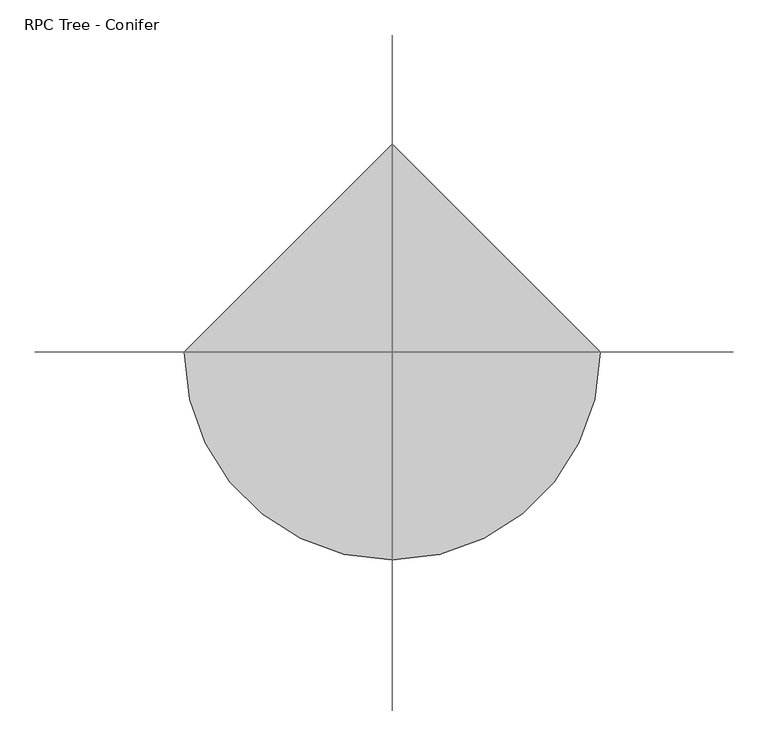
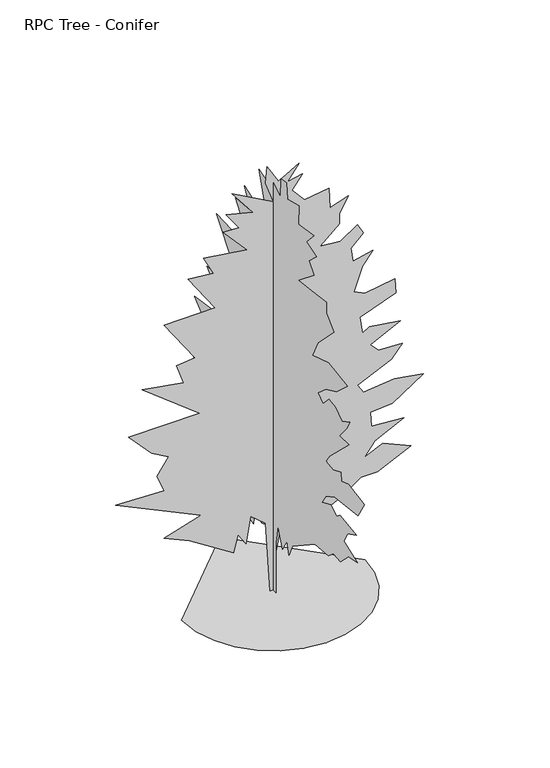
"""IFC4 building model written with IfcOpenShell, lengths in millimetres: geographic element geometry, RPC Tree - Conifer."""

from ifc_helpers import new_model, si_unit, origin, place, context, project, spatial, triangles, source, transform, mapped, element, save


def rpc_tree_conifer_331a7903(model_context):
    return source(origin(), model_context, "Body", "Tessellation", [
        triangles([(-1244.9378185, 0.0, 0.000156), (-1212.0218771, -285.3031886, 0.000156), (-1118.2729483, -547.3069273, 0.000156), (-971.2017654, -778.5080767, 0.000156), (-778.3114317, -971.3984104, 0.000156), (-547.110246, -1118.4695932, 0.000156), (-285.1065255, -1212.2185221, 0.000156), (0.1967255, -1245.1344635, 0.000156), (285.4998518, -1212.2185221, 0.000156), (547.5036086, -1118.4695932, 0.000156), (778.7047216, -971.3984104, 0.000156), (971.5950554, -778.5080767, 0.000156), (1118.6662382, -547.3069273, 0.000156), (1212.415167, -285.3031886, 0.000156), (1245.3311085, 0.0001089, 0.000156), (0.1965078, 1245.1344635, 0.000156), (-42.5774702, 0.0, 0.0), (-102.4597979, -5.92e-05, 994.0450659), (-306.0589711, -6.92e-05, 1161.713102), (-365.9420892, -4.71e-05, 790.44354), (-473.729587, -5.71e-05, 958.1141922), (-533.6101616, -4.28e-05, 718.5868795), (-1132.4334211, -6.57e-05, 1101.8325274), (-1479.7508114, -7.5e-05, 1257.5245502), (-976.7389275, -8.42e-05, 1413.2189713), (-2138.4546455, -0.0001171, 1964.1353439), (-1479.7508114, -0.0001156, 1940.1830269), (-1575.5622597, -0.0001299, 2179.7104122), (-1419.8676933, -0.0001435, 2407.2641098), (-1647.4189201, -0.0001513, 2539.003743), (-1958.8079075, -0.0001713, 2874.3425766), (-1000.6937153, -0.000172, 2886.3313797), (-1779.1611694, -0.0002084, 3497.1254929), (-1216.2687836, -0.0002027, 3401.316806), (-1312.0802319, -0.0002192, 3676.7546448), (-1060.5742172, -0.0002206, 3700.7066711), (-1479.7508114, -0.000257, 4311.5263641), (-785.1161036, -0.0002577, 4323.4898781), (-1156.3856655, -0.0002898, 4862.4276215), (-809.0683479, -0.0002877, 4826.5117905), (-940.8105972, -0.0003034, 5089.9864059), (-353.965967, -0.0002984, 5006.1409424), (-677.3285694, -0.0003198, 5365.4492432), (-461.7535011, -0.0003191, 5353.4604401), (-641.4002392, -0.0003341, 5604.9718323), (-270.1306772, -0.0003284, 5509.1625641), (-557.5649131, -0.0003505, 5880.4346695), (5.3281353, -0.0003319, 5569.0304214), (-102.4597979, -0.0003498, 5868.4458664), (-78.5068178, -0.0003633, 6096.0046509), (77.186931, -0.0003476, 5832.5306168), (352.6448267, -0.0003576, 6000.1959641), (196.9510597, -0.0003448, 5784.6259827), (400.5492791, -0.0003476, 5832.5306168), (256.8333966, -0.0003362, 5640.9126617), (424.5040306, -0.0003248, 5449.2697083), (759.8426462, -0.0003277, 5497.173761), (771.8188047, -0.0003105, 5209.7471191), (1023.324674, -0.0003155, 5293.5925827), (903.561054, -0.0003034, 5089.9864059), (903.561054, -0.0002941, 4934.2842819), (640.0790262, -0.0002805, 4706.7507866), (915.5372126, -0.0002791, 4682.7731804), (1143.0883667, -0.0002884, 4838.4753044), (1226.9236565, -0.0002798, 4694.7619835), (1059.2530043, -0.0002698, 4527.0963455), (1083.2077921, -0.0002584, 4335.4786812), (1358.6659058, -0.000262, 4395.3465385), (1214.9475706, -0.0002513, 4215.6920975), (1095.1838779, -0.000232, 3892.3499153), (1250.8784443, -0.0002277, 3820.4932549), (1658.0762638, -0.0002313, 3880.3611122), (1670.0524223, -0.0002192, 3676.7546448), (1179.0192404, -0.0002084, 3497.1254929), (1214.9475706, -0.0001942, 3257.5779053), (1310.7589462, -0.0001977, 3317.4713425), (1729.9355404, -0.0001942, 3257.5779053), (1322.7351048, -0.000182, 3053.996727), (1430.5251823, -0.0001749, 2934.2357231), (1753.8877121, -0.0001742, 2922.24692), (1610.1693043, -0.0001635, 2742.5924789), (1143.0883667, -0.0001513, 2539.003743), (1226.9236565, -0.0001435, 2407.2641098), (1646.1002506, -0.0001463, 2455.1684532), (2041.3219116, -0.0001421, 2383.309322), (1622.1454628, -0.0001256, 2107.8511356), (1322.7351048, -0.0001242, 2083.8989639), (1334.7111179, -0.0001121, 1880.3000542), (1777.8398838, -0.0001099, 1844.3717239), (1382.6182228, -9.85e-05, 1652.7488274), (1238.899815, -8.78e-05, 1473.1020893), (1490.4056843, -9.42e-05, 1580.8896961), (1873.6513321, -8.42e-05, 1413.2189713), (1418.5464077, -7.14e-05, 1197.6439756), (1190.9953262, -7.14e-05, 1197.6439756), (915.5372126, -6e-05, 1006.0211517), (652.0551121, -5.14e-05, 862.3027439), (520.3154426, -4.43e-05, 742.5391239), (304.7378308, -5.21e-05, 874.2788298), (232.8804073, -4.07e-05, 682.6560059), (113.1160152, -5.5e-05, 922.185862), (29.2812182, -2.78e-05, 467.0809739), (41.2573291, 0.0, 0.0), (0.1966711, 53.1142362, 0.000156), (0.1966711, 89.0438381, 646.7276756), (0.1966711, 112.9965639, 850.3266581), (0.1966711, 268.6890319, 802.4221693), (0.1966711, 424.3835438, 934.1619478), (0.1966711, 460.311874, 670.67992), (0.1966711, 963.3236853, 802.4221693), (0.1966711, 1574.1204872, 1149.7370161), (0.1966711, 1166.9226677, 1341.35984), (0.1966711, 1765.7433838, 1676.7009991), (0.1966711, 1238.7817989, 1808.4407776), (0.1966711, 1897.4856331, 2227.6173717), (0.1966711, 1466.3330257, 2287.5004898), (0.1966711, 1645.9797638, 2550.9748146), (0.1966711, 1310.6410755, 2634.8202782), (0.1966711, 1849.5786736, 3089.912558), (0.1966711, 1047.1590477, 3209.6735619), (0.1966711, 1550.1683155, 3700.7066711), (0.1966711, 1107.0395496, 3724.6589882), (0.1966711, 1202.8509979, 4048.0267502), (0.1966711, 939.3715136, 4107.9198967), (0.1966711, 1334.5932472, 4586.9642029), (0.1966711, 484.2666255, 4551.0486626), (0.1966711, 879.4883955, 5089.9864059), (0.1966711, 532.1710779, 5113.9384323), (0.1966711, 675.8894857, 5389.4018509), (0.1966711, 112.9965639, 5197.7838959), (0.1966711, 184.8552501, 5413.3538773), (0.1966711, 328.5721318, 5832.5306168), (0.1966711, 89.0438381, 5760.6739563), (0.1966711, 124.9729223, 5928.3393036), (0.1966711, -174.437681, 5748.6851532), (0.1966711, -186.4143119, 6012.1591873), (0.1966711, -318.1555801, 6036.111795), (0.1966711, -342.1077882, 5808.578009), (0.1966711, -605.589816, 5880.4346695), (0.1966711, -593.6137301, 5604.9718323), (0.1966711, -964.8832558, 5664.8646881), (0.1966711, -785.2365177, 5473.2217346), (0.1966711, -1024.7638304, 5401.3650742), (0.1966711, -845.1170923, 5233.6997269), (0.1966711, -964.8832558, 5101.9496292), (0.1966711, -593.6137301, 4802.5597641), (0.1966711, -952.9071699, 4850.4641075), (0.1966711, -1252.3174553, 4886.3796478), (0.1966711, -1252.3174553, 4730.7031036), (0.1966711, -1431.9641933, 4563.0121765), (0.1966711, -1060.6947041, 4191.7400711), (0.1966711, -928.9523821, 3928.2654556), (0.1966711, -1300.221944, 4048.0267502), (0.1966711, -1755.3268684, 3988.1588928), (0.1966711, -1491.8448406, 3748.6365944), (0.1966711, -1240.3414421, 3628.8500107), (0.1966711, -1060.6947041, 3473.1734665), (0.1966711, -1168.4822382, 3377.364489), (0.1966711, -1312.1981026, 3533.0413239), (0.1966711, -1467.8925236, 3509.0890068), (0.1966711, -1623.5870899, 3401.316806), (0.1966711, -1803.233828, 3497.1254929), (0.1966711, -1731.3745514, 3365.3756859), (0.1966711, -1563.7039719, 3161.7692184), (0.1966711, -1779.2790401, 3161.7692184), (0.1966711, -1324.1767319, 2718.6404526), (0.1966711, -1240.3414421, 2598.879158), (0.1966711, -1408.0095509, 2574.9271317), (0.1966711, -1599.6323021, 2658.7725952), (0.1966711, -1611.6109314, 2539.003743), (0.1966711, -1767.3028816, 2586.9159348), (0.1966711, -2150.5485294, 2527.0277298), (0.1966711, -1994.8565792, 2275.5217152), (0.1966711, -1455.9165104, 2215.6412132), (0.1966711, -1240.3414421, 2095.8751225), (0.1966711, -1144.5299938, 1952.1591854), (0.1966711, -1360.1050621, 2047.9706337), (0.1966711, -1491.8448406, 1964.1353439), (0.1966711, -1575.6801304, 2024.018462), (0.1966711, -1958.9257782, 1976.1113571), (0.1966711, -1755.3268684, 1868.3238956), (0.1966711, -1671.4915787, 1712.6293293), (0.1966711, -1982.880566, 1592.8657093), (0.1966711, -1767.3028816, 1544.9613659), (0.1966711, -1587.6561436, 1365.3146278), (0.1966711, -1419.9881802, 1377.290641), (0.1966711, -1300.221944, 1281.4793381), (0.1966711, -988.8355001, 1257.5245502), (0.1966711, -461.8714445, 910.2097034), (0.1966711, -378.0361184, 730.5630381), (0.1966711, -330.131666, 898.2336176), (0.1966711, -222.343387, 718.5868795), (0.1966711, -114.5556167, 994.0450659), (0.1966711, -66.6499061, 718.5868795), (0.1966711, -66.6499061, 0.000156)], [[15, 16, 1], [14, 15, 1], [14, 1, 2], [13, 14, 2], [13, 2, 3], [13, 3, 4], [12, 13, 4], [11, 12, 4], [11, 4, 5], [11, 5, 6], [11, 6, 7], [11, 7, 8], [11, 8, 9], [11, 9, 10], [51, 52, 53], [25, 26, 27], [46, 47, 48], [32, 33, 34], [88, 89, 90], [76, 77, 78], [49, 50, 51], [67, 68, 69], [53, 54, 55], [44, 45, 46], [58, 59, 60], [23, 24, 25], [19, 20, 21], [84, 85, 86], [42, 43, 44], [99, 100, 101], [30, 31, 32], [92, 93, 94], [38, 39, 40], [79, 80, 81], [40, 41, 42], [91, 92, 94], [36, 37, 38], [91, 94, 95], [29, 30, 32], [48, 49, 51], [75, 76, 78], [79, 81, 82], [21, 22, 23], [102, 103, 17], [102, 17, 18], [101, 102, 18], [21, 23, 25], [34, 35, 36], [83, 84, 86], [83, 86, 87], [48, 51, 53], [48, 53, 55], [56, 57, 58], [71, 72, 73], [71, 73, 74], [63, 64, 65], [63, 65, 66], [19, 21, 25], [78, 79, 82], [70, 71, 74], [97, 98, 99], [38, 40, 42], [42, 44, 46], [42, 46, 48], [67, 69, 70], [48, 55, 56], [42, 48, 56], [42, 56, 58], [27, 28, 29], [42, 58, 60], [42, 60, 61], [42, 61, 62], [38, 42, 62], [36, 38, 62], [25, 27, 29], [25, 29, 32], [19, 25, 32], [88, 90, 91], [32, 34, 36], [32, 36, 62], [19, 32, 62], [19, 62, 63], [19, 63, 66], [19, 66, 67], [19, 67, 70], [19, 70, 74], [19, 74, 75], [19, 75, 78], [19, 78, 82], [19, 82, 83], [19, 83, 87], [19, 87, 88], [19, 88, 91], [18, 19, 91], [101, 18, 91], [99, 101, 91], [97, 99, 91], [96, 97, 91], [95, 96, 91], [161, 162, 163], [182, 183, 184], [179, 180, 181], [140, 141, 142], [114, 115, 116], [189, 190, 191], [112, 113, 114], [128, 129, 130], [164, 165, 166], [133, 134, 135], [120, 121, 122], [124, 125, 126], [118, 119, 120], [153, 154, 155], [191, 192, 193], [131, 132, 133], [110, 111, 112], [126, 127, 128], [142, 143, 144], [171, 172, 173], [171, 173, 174], [170, 171, 174], [161, 163, 164], [116, 117, 118], [168, 169, 170], [138, 139, 140], [168, 170, 174], [153, 155, 156], [152, 153, 156], [108, 109, 110], [147, 148, 149], [152, 156, 157], [136, 137, 138], [135, 136, 138], [122, 123, 124], [144, 145, 146], [149, 150, 151], [194, 195, 104], [194, 104, 105], [194, 105, 106], [193, 194, 106], [147, 149, 151], [146, 147, 151], [126, 128, 130], [108, 110, 112], [179, 181, 182], [178, 179, 182], [131, 133, 135], [182, 184, 185], [182, 185, 186], [167, 168, 174], [167, 174, 175], [178, 182, 186], [160, 161, 164], [159, 160, 164], [158, 159, 164], [158, 164, 166], [130, 131, 135], [177, 178, 186], [176, 177, 186], [176, 186, 187], [176, 187, 188], [146, 151, 152], [135, 138, 140], [130, 135, 140], [130, 140, 142], [130, 142, 144], [130, 144, 146], [126, 130, 146], [126, 146, 152], [124, 126, 152], [122, 124, 152], [120, 122, 152], [120, 152, 157], [118, 120, 157], [118, 157, 158], [118, 158, 166], [118, 166, 167], [118, 167, 175], [118, 175, 176], [118, 176, 188], [118, 188, 189], [118, 189, 191], [118, 191, 193], [116, 118, 193], [114, 116, 193], [112, 114, 193], [108, 112, 193], [108, 193, 106], [107, 108, 106]], closed=False),
    ])


if __name__ == "__main__":
    model = new_model("IFC4")
    model_context = context("Model", 3, world=origin())
    ifc_project = project(units=[si_unit("LENGTHUNIT", "METRE", prefix="MILLI")], contexts=[model_context])
    site = spatial("IfcSite", under=ifc_project)
    building = spatial("IfcBuilding", under=site)
    placement = place(None, origin())
    rpc_tree_conifer_shape = rpc_tree_conifer_331a7903(model_context)
    element("IfcGeographicElement", 1, ObjectType="RPC Tree - Conifer", at=placement, inside=building, context=model_context, shape_type="MappedRepresentation", body=[
        mapped(rpc_tree_conifer_shape, transform((0.0, 0.0, 0.0), x_axis=(1.0, 0.0, 0.0), y_axis=(0.0, 1.0, 0.0), z_axis=(0.0, 0.0, 1.0))),
    ])
    save(model, "model.ifc")

# Revit data of these elements
# Type "RPC Tree - Conifer"
#   built-in parameter 1005195 = "RPC-16-FVGW-AKQ0-7N2K-N000-ST1L-LVER-AU"
#   Assembly Code = "G2050500"
#   Height = 20' - 0"
#   Description = (empty or 0)
#   Default Elevation = 0
